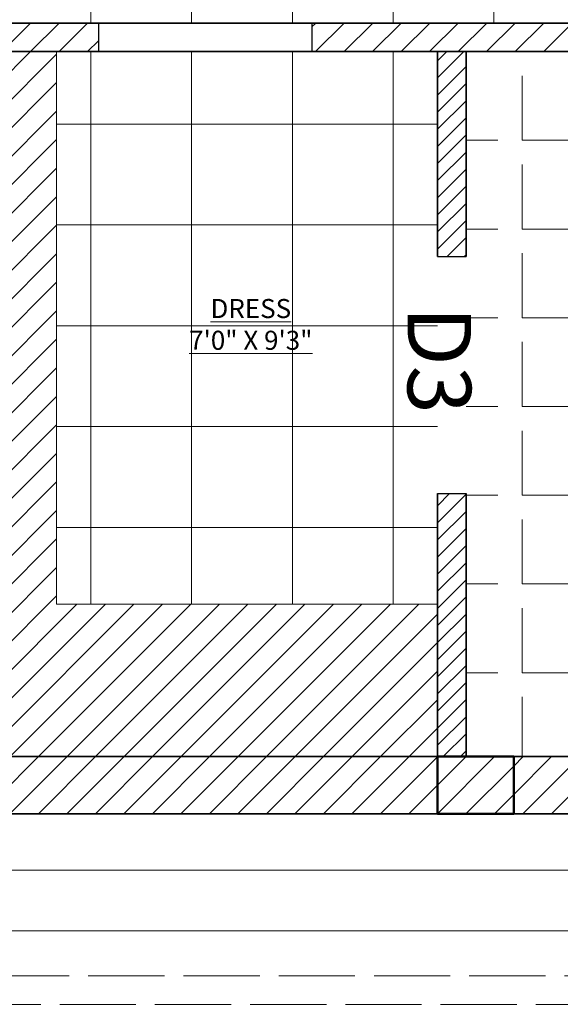
# Model space of a CAD drawing. Units: inches. Extents: x 2036 to 2670, y 319 to 920.
# Tile 12 of 15: x 2449 to 2535, y 465 to 620. Entities that reach past the tile are written whole.
import ezdxf

# ---------------------------------------------------------------- set-up
doc = ezdxf.new("R2010")
doc.units = ezdxf.units.IN
doc.linetypes.add('ACAD_ISO02W100', pattern=[15, 12, -3])
for name, color, linetype, lineweight in [('A-ANNO-DIMS', 2, 'Continuous', 18), ('A-ANNO-TEXT', 7, 'Continuous', 18), ('A-AREA-IDEN', 7, 'Continuous', 18), ('A-CASE', 7, 'Continuous', 18), ('A-CASE-PATT', 9, 'Continuous', 13), ('A-COLS', 7, 'Continuous', 50), ('A-DOOR', 3, 'Continuous', 25), ('A-FLOR-OVHD', 1, 'ACAD_ISO02W100', 13), ('A-FLOR-PATT', 8, 'Continuous', 9), ('A-WALL', 7, 'Continuous', 35)]:
    doc.layers.add(name, color=color, linetype=linetype, lineweight=lineweight)
doc.layers.add('A-COLS-PATT', color=240, linetype='Continuous', lineweight=13, true_color=0xed1f24)
doc.layers.add('A-WALL-PATT', color=52, linetype='Continuous', lineweight=13, true_color=0xc8c92d)
doc.styles.get("Standard").update_dxf_attribs({"font": 'arial.ttf'})
doc.dimstyles.new('ISO-25', dxfattribs={"dimtxt": 10, "dimasz": 6, "dimexe": 1.25, "dimexo": 0.625, "dimtad": 0, "dimdec": 1, "dimlunit": 3, "dimtxsty": 'Standard', "dimblk": 'OBLIQUE', "dimcen": 2.5, "dimclrd": 94, "dimclre": 94, "dimclrt": 1, "dimadec": 0, "dimazin": 0, "dimtfac": 1, "dimtdec": 1, "dimtmove": 0, "dimatfit": 3, "dimfxl": 1, "dimfxlon": 1, "dimarcsym": 0})

# ---------------------------------------------------------------- blocks, each defined once
blk = doc.blocks.new('COL-9x12')
blk.add_lwpolyline([(9, 0), (0, 0), (0, 12), (9, 12)], close=True)
blk = doc.blocks.new('_Oblique')
at = {"color": 0, "linetype": 'ByBlock', "lineweight": -2}
blk.add_line((-0.5, -0.5), (0.5, 0.5), dxfattribs=at)
blk = doc.blocks.new('*D54')
at = {"layer": 'A-ANNO-DIMS', "color": 94, "lineweight": -2, "transparency": 16777216}
for p, q in [((2642.09, 545.51), (2642.09, 551.51)), ((2641.09, 545.51), (2643.34, 545.51)), ((2642.09, 513.19), (2642.09, 545.51)), ((2641.09, 513.19), (2643.34, 513.19))]:
    blk.add_line(p, q, dxfattribs=at)
at = {"layer": 'Defpoints', "color": 0, "transparency": 16777216}
for p in [(2158.74, 545.51), (2642.09, 545.51), (2158.74, 513.19)]:
    blk.add_point(p, dxfattribs=at)
at = {"layer": 'A-ANNO-DIMS', "color": 94, "lineweight": -2, "transparency": 16777216, "xscale": 6, "yscale": 6, "zscale": 6}
for p, rotation in [((2642.09, 545.51), 90), ((2642.09, 513.19), 270)]:
    blk.add_blockref('_Oblique', p, dxfattribs=dict(at, rotation=rotation))
at = {"layer": 'A-ANNO-DIMS', "color": 1, "transparency": 16777216, "insert": (2642.09, 577.16), "char_height": 10, "attachment_point": 5, "rotation": 90}
blk.add_mtext('2\'-8 1/2"', dxfattribs=at)
blk = doc.blocks.new('*D55')
at = {"layer": 'A-ANNO-DIMS', "color": 94, "lineweight": -2, "transparency": 16777216}
for p, q in [((2641.09, 582.53), (2643.34, 582.53)), ((2642.09, 582.53), (2642.09, 577.94)), ((2642.09, 545.51), (2642.09, 550.11)), ((2641.09, 545.51), (2643.34, 545.51))]:
    blk.add_line(p, q, dxfattribs=at)
at = {"layer": 'Defpoints', "color": 0, "transparency": 16777216}
for p in [(2158.74, 582.53), (2642.09, 582.53), (2158.74, 545.51)]:
    blk.add_point(p, dxfattribs=at)
at = {"layer": 'A-ANNO-DIMS', "color": 94, "lineweight": -2, "transparency": 16777216, "xscale": 6, "yscale": 6, "zscale": 6}
for p, rotation in [((2642.09, 582.53), 90), ((2642.09, 545.51), 270)]:
    blk.add_blockref('_Oblique', p, dxfattribs=dict(at, rotation=rotation))
at = {"layer": 'A-ANNO-DIMS', "color": 1, "transparency": 16777216, "insert": (2642.09, 564.02), "char_height": 10, "attachment_point": 5, "rotation": 90}
blk.add_mtext('3\'-1"', dxfattribs=at)
blk = doc.blocks.new('*D56')
at = {"layer": 'A-ANNO-DIMS', "color": 94, "lineweight": -2, "transparency": 16777216}
for p, q in [((2642.09, 599.85), (2642.09, 605.85)), ((2641.09, 599.85), (2643.34, 599.85)), ((2642.09, 582.53), (2642.09, 599.85)), ((2641.09, 582.53), (2643.34, 582.53))]:
    blk.add_line(p, q, dxfattribs=at)
at = {"layer": 'Defpoints', "color": 0, "transparency": 16777216}
for p in [(2158.74, 599.85), (2642.09, 599.85), (2158.74, 582.53)]:
    blk.add_point(p, dxfattribs=at)
at = {"layer": 'A-ANNO-DIMS', "color": 94, "lineweight": -2, "transparency": 16777216, "xscale": 6, "yscale": 6, "zscale": 6}
for p, rotation in [((2642.09, 599.85), 90), ((2642.09, 582.53), 270)]:
    blk.add_blockref('_Oblique', p, dxfattribs=dict(at, rotation=rotation))
at = {"layer": 'A-ANNO-DIMS', "color": 1, "transparency": 16777216, "insert": (2642.09, 630.95), "char_height": 10, "attachment_point": 5, "rotation": 90}
blk.add_mtext('1\'-5 1/2"', dxfattribs=at)
blk = doc.blocks.new('*D60')
at = {"layer": 'A-ANNO-DIMS', "color": 94, "lineweight": -2, "transparency": 16777216}
for p, q in [((2051.39, 582.41), (2051.39, 588.41)), ((2052.39, 582.41), (2050.14, 582.41)), ((2051.39, 545.09), (2051.39, 582.41)), ((2052.39, 545.09), (2050.14, 545.09))]:
    blk.add_line(p, q, dxfattribs=at)
at = {"layer": 'Defpoints', "color": 0, "transparency": 16777216}
for p in [(2051.39, 582.41), (2515.24, 582.41), (2515.24, 545.09)]:
    blk.add_point(p, dxfattribs=at)
at = {"layer": 'A-ANNO-DIMS', "color": 94, "lineweight": -2, "transparency": 16777216, "xscale": 6, "yscale": 6, "zscale": 6}
for p, rotation in [((2051.39, 582.41), 90), ((2051.39, 545.09), 270)]:
    blk.add_blockref('_Oblique', p, dxfattribs=dict(at, rotation=rotation))
at = {"layer": 'A-ANNO-DIMS', "color": 1, "transparency": 16777216, "insert": (2051.39, 613.98), "char_height": 10, "attachment_point": 5, "rotation": 90}
blk.add_mtext('3\'-1 1/2"', dxfattribs=at)

msp = doc.modelspace()

# ---------------------------------------------------------------- hatches: boundary and pattern name
at = {"layer": 'A-CASE-PATT'}
h = msp.add_hatch(dxfattribs=at)
h.set_pattern_fill('ANSI31', color=256)
h.paths.add_polyline_path([(2455.24, 614.68), (2431.24, 614.68), (2431.24, 503.68), (2515.24, 503.68), (2515.24, 527.68), (2455.24, 527.68)])
at = {"layer": 'A-COLS-PATT'}
h = msp.add_hatch(dxfattribs=at)
h.set_pattern_fill('ANSI31', color=256)
h.paths.add_polyline_path([(2089.74, 875.68), (2080.74, 875.68), (2080.74, 863.68), (2089.74, 863.68)])
h.paths.add_polyline_path([(2089.74, 821.68), (2080.74, 821.68), (2080.74, 809.68), (2089.74, 809.68)])
h.paths.add_polyline_path([(2089.74, 624.2), (2080.74, 624.2), (2080.74, 612.2), (2089.74, 612.2)])
h.paths.add_polyline_path([(2158.74, 506.68), (2149.74, 506.68), (2149.74, 494.68), (2158.74, 494.68)])
h.paths.add_polyline_path([(2158.74, 617.33), (2149.74, 617.33), (2149.74, 605.33), (2158.74, 605.33)])
h.paths.add_polyline_path([(2158.74, 736.18), (2149.74, 736.18), (2149.74, 724.18), (2158.74, 724.18)])
h.paths.add_polyline_path([(2158.74, 852.81), (2149.74, 852.81), (2149.74, 843.81), (2158.74, 843.81)])
h.paths.add_polyline_path([(2161.74, 852.81), (2158.74, 852.81), (2158.74, 843.81), (2161.74, 843.81)])
h.paths.add_polyline_path([(2295.21, 857.66), (2290.74, 857.66), (2290.74, 848.68), (2295.21, 848.68)])
h.paths.add_polyline_path([(2290.74, 857.66), (2283.21, 857.66), (2283.21, 848.66), (2290.74, 848.66)])
h.paths.add_polyline_path([(2443.62, 857.68), (2431.62, 857.68), (2431.62, 848.68), (2443.62, 848.68)])
h.paths.add_polyline_path([(2561.81, 857.68), (2549.81, 857.68), (2549.81, 848.68), (2561.81, 848.68)])
h.paths.add_polyline_path([(2295.24, 737.65), (2290.74, 737.65), (2290.74, 728.68), (2295.24, 728.68)])
h.paths.add_polyline_path([(2309.27, 612.12), (2297.27, 612.12), (2297.27, 603.12), (2309.27, 603.12)])
h.paths.add_polyline_path([(2282.24, 503.68), (2270.24, 503.68), (2270.24, 494.68), (2282.24, 494.68)])
h.paths.add_polyline_path([(2431.74, 746.09), (2427.24, 746.09), (2427.24, 737.09), (2431.74, 737.09)])
h.paths.add_polyline_path([(2439.24, 746.09), (2431.74, 746.09), (2431.74, 737.09), (2439.24, 737.09)])
h.paths.add_polyline_path([(2596.59, 736.59), (2584.59, 736.59), (2584.59, 727.59), (2596.59, 727.59)])
h.paths.add_polyline_path([(2586.39, 623.71), (2574.39, 623.71), (2574.39, 619.18), (2586.39, 619.18)])
h.paths.add_polyline_path([(2586.39, 619.18), (2574.39, 619.18), (2574.39, 614.71), (2586.39, 614.71)])
h.paths.add_polyline_path([(2438.74, 623.68), (2431.24, 623.68), (2431.24, 619.18), (2438.74, 619.18)])
h.paths.add_polyline_path([(2438.74, 619.18), (2431.24, 619.18), (2431.24, 614.68), (2438.74, 614.68)])
h.paths.add_polyline_path([(2431.24, 623.68), (2426.74, 623.68), (2426.74, 614.68), (2431.24, 614.68), (2431.24, 619.18)])
h.paths.add_polyline_path([(2527.24, 503.68), (2515.24, 503.68), (2515.24, 494.68), (2527.24, 494.68)])
h.paths.add_polyline_path([(2590.31, 503.68), (2578.31, 503.68), (2578.31, 494.68), (2590.31, 494.68)])
at = {"layer": 'A-FLOR-PATT'}
h = msp.add_hatch(dxfattribs=at)
h.set_pattern_fill('ANSI31', color=256, scale=5, angle=135)
h.paths.add_polyline_path([(2290.74, 659.68), (2158.74, 659.68), (2158.74, 582.53), (2158.74, 545.51), (2158.74, 503.68), (2426.74, 503.68), (2426.74, 614.68), (2426.74, 623.68), (2426.74, 628.18), (2431.24, 628.18), (2431.24, 623.68), (2438.74, 623.68), (2438.74, 619.18), (2574.39, 619.18), (2574.39, 623.71), (2586.39, 623.71), (2586.39, 619.18), (2603.74, 619.18), (2603.74, 824.68), (2431.74, 824.68), (2431.74, 746.09), (2439.24, 746.09), (2439.24, 737.09), (2431.74, 737.09), (2431.74, 659.68), (2427.24, 659.68), (2427.24, 739.48), (2383.24, 739.48), (2383.24, 804.68), (2339.24, 804.68), (2339.24, 749.08), (2295.24, 749.08), (2295.24, 737.65), (2295.27, 737.65), (2295.27, 728.65), (2295.21, 728.65, -0.586418), (2272.74, 728.68), (2272.74, 824.68), (2270.11, 824.68), (2270.11, 829.18), (2290.74, 829.18), (2290.74, 848.66), (2283.21, 848.66), (2283.21, 857.66), (2289.74, 857.66), (2289.74, 874.68), (2158.74, 874.68), (2158.74, 852.81), (2161.74, 852.81), (2161.74, 843.81), (2158.74, 843.81), (2158.74, 829.18), (2224.74, 829.18), (2224.74, 800.68), (2182.74, 800.68), (2182.74, 733.41), (2158.74, 733.41), (2158.74, 728.68), (2235.24, 728.68), (2235.24, 714.81), (2230.74, 714.81), (2230.74, 724.18), (2158.74, 724.18), (2158.74, 664.18), (2230.74, 664.18), (2230.74, 678.81), (2235.24, 678.81), (2235.24, 664.18), (2290.74, 664.18)])
h.paths.add_polyline_path([(2309.27, 612.12), (2309.27, 603.12), (2297.27, 603.12), (2297.27, 612.12)], flags=16)
h.paths.add_polyline_path([(2280.12, 639.11), (2280.26, 638.18, -0.414214), (2279.26, 637.18), (2278.76, 637.18), (2279.26, 633.18), (2277.76, 633.18), (2277.26, 637.18), (2269.76, 637.18), (2262.26, 637.18), (2261.76, 633.18), (2260.26, 633.18), (2260.76, 637.18), (2260.26, 637.18, -0.414214), (2259.26, 638.18), (2259.41, 639.11, -0.541164), (2257.76, 641.18), (2260.76, 652.18), (2261.45, 652.18), (2261.53, 652.68), (2262.76, 652.68), (2262.25, 655.24, 0.001913), (2261.76, 655.18), (2259.76, 658.18, -0.15), (2279.76, 658.18), (2277.76, 655.18, 0.001913), (2277.27, 655.24), (2276.76, 652.68), (2278, 652.68), (2278.07, 652.18), (2278.76, 652.18), (2281.76, 641.18, -0.541163)], flags=16)
h.paths.add_polyline_path([(2245.98, 639.11), (2246.13, 638.18, -0.414214), (2245.13, 637.18), (2244.63, 637.18), (2245.13, 633.18), (2243.63, 633.18), (2243.13, 637.18), (2235.63, 637.18), (2228.13, 637.18), (2227.63, 633.18), (2226.13, 633.18), (2226.63, 637.18), (2226.13, 637.18, -0.414214), (2225.13, 638.18), (2225.27, 639.11, -0.541164), (2223.63, 641.18), (2226.63, 652.18), (2227.32, 652.18), (2227.39, 652.68), (2228.63, 652.68), (2228.12, 655.24, 0.001913), (2227.63, 655.18), (2225.63, 658.18, -0.15), (2245.63, 658.18), (2243.63, 655.18, 0.001913), (2243.14, 655.24), (2242.63, 652.68), (2243.86, 652.68), (2243.94, 652.18), (2244.63, 652.18), (2247.63, 641.18, -0.541163)], flags=16)
h.paths.add_polyline_path([(2351.59, 515.15, -0.151948), (2279.59, 515.15), (2279.59, 537.68), (2273.59, 537.68), (2273.59, 511.68, 0.190476), (2357.59, 511.68), (2357.59, 537.68), (2351.59, 537.68)])
h.paths.add_polyline_path([(2327.59, 536.13), (2327.59, 517.07), (2303.59, 517.07), (2303.59, 536.13)], flags=16)
h.paths.add_polyline_path([(2213.4, 639.11), (2213.55, 638.18, -0.414214), (2212.55, 637.18), (2212.05, 637.18), (2212.55, 633.18), (2211.05, 633.18), (2210.55, 637.18), (2203.05, 637.18), (2195.55, 637.18), (2195.05, 633.18), (2193.55, 633.18), (2194.05, 637.18), (2193.55, 637.18, -0.414214), (2192.55, 638.18), (2192.69, 639.11, -0.541164), (2191.05, 641.18), (2194.05, 652.18), (2194.73, 652.18), (2194.81, 652.68), (2196.05, 652.68), (2195.53, 655.24, 0.001913), (2195.05, 655.18), (2193.05, 658.18, -0.15), (2213.05, 658.18), (2211.05, 655.18, 0.001913), (2210.56, 655.24), (2210.05, 652.68), (2211.28, 652.68), (2211.36, 652.18), (2212.05, 652.18), (2215.05, 641.18, -0.541163)], flags=16)
h.paths.add_polyline_path([(2368.58, 538.02), (2370.52, 538.02), (2371.17, 532.84), (2380.89, 532.84), (2390.6, 532.84), (2391.25, 538.02), (2393.2, 538.02), (2392.55, 532.84), (2380.89, 532.84), (2368.58, 532.84, 0.414214), (2367.28, 531.54), (2367.47, 530.34, -0.483352), (2369.23, 527.65), (2371.82, 513.4), (2370.12, 513.4), (2370.22, 512.75), (2391.56, 512.75), (2391.66, 513.4), (2389.96, 513.4), (2392.55, 527.65, -1.387427), (2396.43, 527.65), (2392.55, 513.4), (2391.66, 513.4), (2391.56, 512.75), (2389.31, 512.75), (2390, 509.37, 0.003796), (2391.25, 509.51), (2393.84, 505.63, -0.15), (2367.93, 505.63), (2370.52, 509.51, 0.003901), (2371.81, 509.36), (2372.47, 512.75), (2370.22, 512.75), (2370.12, 513.4), (2369.23, 513.4), (2365.34, 527.65, -0.541163), (2367.47, 530.34), (2367.28, 531.54, -0.414214), (2368.58, 532.84), (2369.23, 532.84)])
h.paths.add_polyline_path([(2266.74, 538.02), (2266.09, 532.84), (2254.43, 532.84), (2242.12, 532.84, 0.414214), (2240.83, 531.54), (2241.01, 530.34, -0.483352), (2242.77, 527.65), (2245.36, 513.4), (2243.66, 513.4), (2243.76, 512.75), (2265.1, 512.75), (2265.2, 513.4), (2263.5, 513.4), (2266.09, 527.65, -1.387427), (2269.98, 527.65), (2266.09, 513.4), (2265.2, 513.4), (2265.1, 512.75), (2262.85, 512.75), (2263.54, 509.37, 0.003796), (2264.79, 509.51), (2267.39, 505.63, -0.15), (2241.47, 505.63), (2244.07, 509.51, 0.003901), (2245.36, 509.36), (2246.01, 512.75), (2243.76, 512.75), (2243.66, 513.4), (2242.77, 513.4), (2238.88, 527.65, -0.541163), (2241.01, 530.34), (2240.83, 531.54, -0.414214), (2242.12, 532.84), (2242.77, 532.84), (2242.12, 538.02), (2244.07, 538.02), (2244.71, 532.84), (2254.43, 532.84), (2264.15, 532.84), (2264.79, 538.02)])
h.paths.add_polyline_path([(2185.24, 620.36), (2185.24, 618.86), (2181.24, 618.36), (2181.24, 610.86), (2181.24, 603.36), (2185.24, 602.86), (2185.24, 601.36), (2181.24, 601.86), (2181.24, 601.36, -0.414214), (2180.24, 600.36), (2179.31, 600.5, -0.541164), (2177.24, 598.86), (2166.24, 601.86), (2166.24, 602.54), (2165.74, 602.62), (2165.74, 603.86), (2163.18, 603.34, 0.001913), (2163.24, 602.86), (2160.24, 600.86, -0.15), (2160.24, 620.86), (2163.24, 618.86, 0.001913), (2163.18, 618.37), (2165.74, 617.86), (2165.74, 619.09), (2166.24, 619.17), (2166.24, 619.86), (2177.24, 622.86, -0.541163), (2179.31, 621.21), (2180.24, 621.36, -0.414214), (2181.24, 620.36), (2181.24, 619.86)])
h.paths.add_polyline_path([(2470.92, 676.01), (2470.92, 806.13), (2568.52, 806.13), (2568.52, 676.01)], flags=16)
h.paths.add_polyline_path([(2177.74, 677.49), (2161.9, 677.49), (2161.9, 705.85), (2177.74, 705.85)], flags=16)
h.paths.add_polyline_path([(2176.74, 678.49), (2162.9, 678.49), (2162.9, 704.85), (2176.74, 704.85)], flags=0)
h.paths.add_polyline_path([(2175.01, 686.48), (2172.93, 686.48), (2172.93, 690.63), (2170.86, 690.63), (2170.86, 686.48), (2164.63, 686.48), (2164.63, 688.56), (2166.71, 688.56), (2168.78, 688.56), (2168.78, 690.63), (2164.63, 690.63), (2164.63, 696.85), (2166.71, 696.85), (2166.71, 692.71), (2168.78, 692.71), (2168.78, 696.85), (2175.01, 696.85), (2175.01, 694.78), (2170.86, 694.78), (2170.86, 692.71), (2175.01, 692.71)], flags=0)
h.paths.add_polyline_path([(2543.79, 782.71), (2483.94, 782.71), (2483.94, 804.18), (2517.77, 804.18), (2517.77, 782.71), (2521.67, 782.71), (2521.67, 804.18), (2555.5, 804.18), (2555.5, 779.45), (2547.05, 779.45), (2568.52, 757.98), (2543.79, 757.98)], flags=0)
h.paths.add_polyline_path([(2584.59, 727.59), (2584.59, 736.59), (2596.59, 736.59), (2596.59, 727.59)], flags=16)
h.paths.add_polyline_path([(2520.45, 647.03), (2553.79, 647.03), (2553.79, 658.23), (2520.45, 658.23)], flags=24)
h.paths.add_polyline_path([(2299.53, 573.74), (2331.71, 573.74), (2331.71, 584.94), (2299.53, 584.94)], flags=24)
h.paths.add_polyline_path([(2191.59, 685.19), (2212.12, 685.19), (2212.12, 696.38), (2191.59, 696.38)], flags=24)
h.paths.add_polyline_path([(2353.9, 649.86), (2379.08, 649.86), (2379.08, 661.06), (2353.9, 661.06)], flags=24)
h.paths.add_polyline_path([(2214.61, 763.31), (2237.46, 763.31), (2237.46, 779.56), (2214.61, 779.56)], flags=24)
h.paths.add_polyline_path([(2225.09, 819.31), (2269.29, 819.31), (2269.29, 844.04), (2225.09, 844.04)], flags=24)
h.paths.add_polyline_path([(2204.06, 845.04), (2226.92, 845.04), (2226.92, 856.24), (2204.06, 856.24)], flags=24)
h = msp.add_hatch(dxfattribs=at)
h.set_pattern_fill('ANSI31', color=256, scale=5, angle=45)
h.paths.add_polyline_path([(2290.74, 659.68), (2158.74, 659.68), (2158.74, 582.53), (2158.74, 545.51), (2158.74, 503.68), (2426.74, 503.68), (2426.74, 614.68), (2426.74, 623.68), (2426.74, 628.18), (2431.24, 628.18), (2431.24, 623.68), (2438.74, 623.68), (2438.74, 619.18), (2574.39, 619.18), (2574.39, 623.71), (2586.39, 623.71), (2586.39, 619.18), (2603.74, 619.18), (2603.74, 824.68), (2431.74, 824.68), (2431.74, 746.09), (2439.24, 746.09), (2439.24, 737.09), (2431.74, 737.09), (2431.74, 659.68), (2427.24, 659.68), (2427.24, 739.48), (2383.24, 739.48), (2383.24, 804.68), (2339.24, 804.68), (2339.24, 749.08), (2295.24, 749.08), (2295.24, 737.65), (2295.27, 737.65), (2295.27, 728.65), (2295.21, 728.65, -0.586418), (2272.74, 728.68), (2272.74, 824.68), (2270.11, 824.68), (2270.11, 829.18), (2290.74, 829.18), (2290.74, 848.66), (2283.21, 848.66), (2283.21, 857.66), (2289.74, 857.66), (2289.74, 874.68), (2158.74, 874.68), (2158.74, 852.81), (2161.74, 852.81), (2161.74, 843.81), (2158.74, 843.81), (2158.74, 829.18), (2224.74, 829.18), (2224.74, 800.68), (2182.74, 800.68), (2182.74, 733.41), (2158.74, 733.41), (2158.74, 728.68), (2235.24, 728.68), (2235.24, 714.81), (2230.74, 714.81), (2230.74, 724.18), (2158.74, 724.18), (2158.74, 664.18), (2230.74, 664.18), (2230.74, 678.81), (2235.24, 678.81), (2235.24, 664.18), (2290.74, 664.18)])
h.paths.add_polyline_path([(2309.27, 612.12), (2309.27, 603.12), (2297.27, 603.12), (2297.27, 612.12)], flags=16)
h.paths.add_polyline_path([(2280.12, 639.11), (2280.26, 638.18, -0.414214), (2279.26, 637.18), (2278.76, 637.18), (2279.26, 633.18), (2277.76, 633.18), (2277.26, 637.18), (2269.76, 637.18), (2262.26, 637.18), (2261.76, 633.18), (2260.26, 633.18), (2260.76, 637.18), (2260.26, 637.18, -0.414214), (2259.26, 638.18), (2259.41, 639.11, -0.541164), (2257.76, 641.18), (2260.76, 652.18), (2261.45, 652.18), (2261.53, 652.68), (2262.76, 652.68), (2262.25, 655.24, 0.001913), (2261.76, 655.18), (2259.76, 658.18, -0.15), (2279.76, 658.18), (2277.76, 655.18, 0.001913), (2277.27, 655.24), (2276.76, 652.68), (2278, 652.68), (2278.07, 652.18), (2278.76, 652.18), (2281.76, 641.18, -0.541163)], flags=16)
h.paths.add_polyline_path([(2245.98, 639.11), (2246.13, 638.18, -0.414214), (2245.13, 637.18), (2244.63, 637.18), (2245.13, 633.18), (2243.63, 633.18), (2243.13, 637.18), (2235.63, 637.18), (2228.13, 637.18), (2227.63, 633.18), (2226.13, 633.18), (2226.63, 637.18), (2226.13, 637.18, -0.414214), (2225.13, 638.18), (2225.27, 639.11, -0.541164), (2223.63, 641.18), (2226.63, 652.18), (2227.32, 652.18), (2227.39, 652.68), (2228.63, 652.68), (2228.12, 655.24, 0.001913), (2227.63, 655.18), (2225.63, 658.18, -0.15), (2245.63, 658.18), (2243.63, 655.18, 0.001913), (2243.14, 655.24), (2242.63, 652.68), (2243.86, 652.68), (2243.94, 652.18), (2244.63, 652.18), (2247.63, 641.18, -0.541163)], flags=16)
h.paths.add_polyline_path([(2351.59, 537.68), (2351.59, 515.15, -0.151948), (2279.59, 515.15), (2279.59, 537.68), (2273.59, 537.68), (2273.59, 511.68, 0.190476), (2357.59, 511.68), (2357.59, 537.68)])
h.paths.add_polyline_path([(2368.58, 538.02), (2370.52, 538.02), (2371.17, 532.84), (2380.89, 532.84), (2390.6, 532.84), (2391.25, 538.02), (2393.2, 538.02), (2392.55, 532.84), (2380.89, 532.84), (2368.58, 532.84, 0.414214), (2367.28, 531.54), (2367.47, 530.34, -0.483352), (2369.23, 527.65), (2371.82, 513.4), (2370.12, 513.4), (2370.22, 512.75), (2391.56, 512.75), (2391.66, 513.4), (2389.96, 513.4), (2392.55, 527.65, -1.387427), (2396.43, 527.65), (2392.55, 513.4), (2391.66, 513.4), (2391.56, 512.75), (2389.31, 512.75), (2390, 509.37, 0.003796), (2391.25, 509.51), (2393.84, 505.63, -0.15), (2367.93, 505.63), (2370.52, 509.51, 0.003901), (2371.81, 509.36), (2372.47, 512.75), (2370.22, 512.75), (2370.12, 513.4), (2369.23, 513.4), (2365.34, 527.65, -0.541163), (2367.47, 530.34), (2367.28, 531.54, -0.414214), (2368.58, 532.84), (2369.23, 532.84)])
h.paths.add_polyline_path([(2327.59, 536.13), (2327.59, 517.07), (2303.59, 517.07), (2303.59, 536.13)], flags=16)
h.paths.add_polyline_path([(2470.92, 676.01), (2470.92, 806.13), (2568.52, 806.13), (2568.52, 676.01)], flags=16)
h.paths.add_polyline_path([(2266.74, 538.02), (2266.09, 532.84), (2254.43, 532.84), (2242.12, 532.84, 0.414214), (2240.83, 531.54), (2241.01, 530.34, -0.483352), (2242.77, 527.65), (2245.36, 513.4), (2243.66, 513.4), (2243.76, 512.75), (2265.1, 512.75), (2265.2, 513.4), (2263.5, 513.4), (2266.09, 527.65, -1.387427), (2269.98, 527.65), (2266.09, 513.4), (2265.2, 513.4), (2265.1, 512.75), (2262.85, 512.75), (2263.54, 509.37, 0.003796), (2264.79, 509.51), (2267.39, 505.63, -0.15), (2241.47, 505.63), (2244.07, 509.51, 0.003901), (2245.36, 509.36), (2246.01, 512.75), (2243.76, 512.75), (2243.66, 513.4), (2242.77, 513.4), (2238.88, 527.65, -0.541163), (2241.01, 530.34), (2240.83, 531.54, -0.414214), (2242.12, 532.84), (2242.77, 532.84), (2242.12, 538.02), (2244.07, 538.02), (2244.71, 532.84), (2254.43, 532.84), (2264.15, 532.84), (2264.79, 538.02)])
h.paths.add_polyline_path([(2213.4, 639.11), (2213.55, 638.18, -0.414214), (2212.55, 637.18), (2212.05, 637.18), (2212.55, 633.18), (2211.05, 633.18), (2210.55, 637.18), (2203.05, 637.18), (2195.55, 637.18), (2195.05, 633.18), (2193.55, 633.18), (2194.05, 637.18), (2193.55, 637.18, -0.414214), (2192.55, 638.18), (2192.69, 639.11, -0.541164), (2191.05, 641.18), (2194.05, 652.18), (2194.73, 652.18), (2194.81, 652.68), (2196.05, 652.68), (2195.53, 655.24, 0.001913), (2195.05, 655.18), (2193.05, 658.18, -0.15), (2213.05, 658.18), (2211.05, 655.18, 0.001913), (2210.56, 655.24), (2210.05, 652.68), (2211.28, 652.68), (2211.36, 652.18), (2212.05, 652.18), (2215.05, 641.18, -0.541163)], flags=16)
h.paths.add_polyline_path([(2185.24, 620.36), (2185.24, 618.86), (2181.24, 618.36), (2181.24, 610.86), (2181.24, 603.36), (2185.24, 602.86), (2185.24, 601.36), (2181.24, 601.86), (2181.24, 601.36, -0.414214), (2180.24, 600.36), (2179.31, 600.5, -0.541164), (2177.24, 598.86), (2166.24, 601.86), (2166.24, 602.54), (2165.74, 602.62), (2165.74, 603.86), (2163.18, 603.34, 0.001913), (2163.24, 602.86), (2160.24, 600.86, -0.15), (2160.24, 620.86), (2163.24, 618.86, 0.001913), (2163.18, 618.37), (2165.74, 617.86), (2165.74, 619.09), (2166.24, 619.17), (2166.24, 619.86), (2177.24, 622.86, -0.541163), (2179.31, 621.21), (2180.24, 621.36, -0.414214), (2181.24, 620.36), (2181.24, 619.86)])
h.paths.add_polyline_path([(2177.74, 677.49), (2161.9, 677.49), (2161.9, 705.85), (2177.74, 705.85)], flags=16)
h.paths.add_polyline_path([(2176.74, 678.49), (2162.9, 678.49), (2162.9, 704.85), (2176.74, 704.85)], flags=0)
h.paths.add_polyline_path([(2175.01, 686.48), (2172.93, 686.48), (2172.93, 690.63), (2170.86, 690.63), (2170.86, 686.48), (2164.63, 686.48), (2164.63, 688.56), (2166.71, 688.56), (2168.78, 688.56), (2168.78, 690.63), (2164.63, 690.63), (2164.63, 696.85), (2166.71, 696.85), (2166.71, 692.71), (2168.78, 692.71), (2168.78, 696.85), (2175.01, 696.85), (2175.01, 694.78), (2170.86, 694.78), (2170.86, 692.71), (2175.01, 692.71)], flags=0)
h.paths.add_polyline_path([(2543.79, 782.71), (2483.94, 782.71), (2483.94, 804.18), (2517.77, 804.18), (2517.77, 782.71), (2521.67, 782.71), (2521.67, 804.18), (2555.5, 804.18), (2555.5, 779.45), (2547.05, 779.45), (2568.52, 757.98), (2543.79, 757.98)], flags=0)
h.paths.add_polyline_path([(2584.59, 727.59), (2584.59, 736.59), (2596.59, 736.59), (2596.59, 727.59)], flags=16)
h.paths.add_polyline_path([(2520.45, 647.03), (2553.79, 647.03), (2553.79, 658.23), (2520.45, 658.23)], flags=24)
h.paths.add_polyline_path([(2299.53, 573.74), (2331.71, 573.74), (2331.71, 584.94), (2299.53, 584.94)], flags=24)
h.paths.add_polyline_path([(2191.59, 685.19), (2212.12, 685.19), (2212.12, 696.38), (2191.59, 696.38)], flags=24)
h.paths.add_polyline_path([(2353.9, 649.86), (2379.08, 649.86), (2379.08, 661.06), (2353.9, 661.06)], flags=24)
h.paths.add_polyline_path([(2214.61, 763.31), (2237.46, 763.31), (2237.46, 779.56), (2214.61, 779.56)], flags=24)
h.paths.add_polyline_path([(2225.09, 819.31), (2269.29, 819.31), (2269.29, 844.04), (2225.09, 844.04)], flags=24)
h.paths.add_polyline_path([(2204.06, 845.04), (2226.92, 845.04), (2226.92, 856.24), (2204.06, 856.24)], flags=24)
h = msp.add_hatch(dxfattribs=at)
h.set_pattern_fill('ANSI31', color=256, scale=3, angle=135)
h.paths.add_polyline_path([(2149.74, 582.53), (2149.74, 707.68), (2120.74, 707.68), (2120.74, 599.68, -1), (2118.74, 599.68), (2085.24, 599.68), (2085.24, 506.68), (2089.74, 506.68), (2089.74, 494.68), (2085.24, 494.68), (2085.24, 469.18), (2608.24, 469.18), (2608.24, 494.68), (2149.74, 494.68), (2149.74, 506.68), (2149.74, 545.51)])
h.paths.add_polyline_path([(2143.58, 686.71), (2149.03, 686.71), (2149.03, 692.89), (2143.58, 692.89)], flags=24)
h.paths.add_polyline_path([(2125.99, 700.31), (2133.31, 700.31), (2133.31, 706.49), (2125.99, 706.49)], flags=24)
h = msp.add_hatch(dxfattribs=at)
h.set_pattern_fill('ANSI31', color=256, scale=5, angle=45)
h.paths.add_polyline_path([(2515.24, 614.68), (2455.24, 614.68), (2455.24, 527.68), (2515.24, 527.68)])
h.paths.add_polyline_path([(2475.58, 566.03), (2496.1, 566.03), (2496.1, 577.23), (2475.58, 577.23)], flags=24)
h = msp.add_hatch(dxfattribs=at)
h.set_pattern_fill('ANSI31', color=256, scale=5, angle=135)
h.paths.add_polyline_path([(2515.24, 614.68), (2455.24, 614.68), (2455.24, 527.68), (2515.24, 527.68)])
h.paths.add_polyline_path([(2475.58, 566.03), (2496.1, 566.03), (2496.1, 577.23), (2475.58, 577.23)], flags=24)
h = msp.add_hatch(dxfattribs=at)
h.set_pattern_fill('ANGLE', color=256, scale=2)
h.set_pattern_definition([(0, (0, 0), (0, 13.97), [10.16, -3.81]), (90, (0, 0), (-13.97, 9e-16), [10.16, -3.81])])
h.paths.add_polyline_path([(2519.74, 503.68), (2527.24, 503.68), (2603.74, 503.68), (2603.74, 614.68), (2519.74, 614.68)])
h.paths.add_polyline_path([(2569.98, 598.38), (2571.98, 604.38), (2568.98, 604.38), (2568.98, 602.88), (2565.98, 602.88), (2565.98, 603.88), (2567.98, 603.88), (2567.98, 604.38), (2565.48, 604.38), (2565.48, 612.38), (2586.48, 612.38), (2586.48, 604.38), (2579.98, 604.38), (2581.98, 598.38, -0.501323), (2577.03, 579.52, -0.132891), (2574.94, 579.52, -0.501317)], flags=16)
h.paths.add_polyline_path([(2571.98, 598.38), (2579.98, 598.38, -0.48008), (2577.63, 580.86, -0.215004), (2574.34, 580.86, -0.48008)], flags=0)
h.paths.add_polyline_path([(2546.37, 611.78), (2546.37, 613.08), (2543.76, 613.08), (2543.76, 611.78)], flags=16)
h.paths.add_polyline_path([(2543.76, 609.82), (2544.41, 609.82), (2544.41, 611.13), (2545.72, 611.13), (2545.72, 609.82), (2554.18, 609.82, -0.293434), (2556.79, 605.92), (2554.18, 605.92, 0.553806), (2552.88, 607.22), (2546.37, 607.22), (2546.37, 606.24), (2547.02, 606.24, -0.791418), (2548.4, 605.92, -0.791418), (2547.02, 605.59), (2546.57, 605.59, -0.086626), (2547.58, 602.73, 0.107048), (2548.97, 602.01), (2541.81, 602.01), (2541.16, 602.01, -0.159443)], flags=16)
h.paths.add_polyline_path([(2542.38, 605.92, -1), (2543.84, 605.92, -1)], flags=0)
h.paths.add_polyline_path([(2544.66, 605.92, -1), (2546.12, 605.92, -1)], flags=0)
h.paths.add_polyline_path([(2566.48, 606.38), (2566.48, 610.38, -0.5), (2567.48, 611.38), (2584.48, 611.38, -0.5), (2585.48, 610.38), (2585.48, 606.38, -0.5), (2584.48, 605.38), (2567.48, 605.38, -0.5)], flags=0)
h.paths.add_polyline_path([(2552.87, 546.2), (2581.15, 546.2), (2581.15, 557.39), (2552.87, 557.39)], flags=24)
at = {"layer": 'A-WALL-PATT'}
h = msp.add_hatch(dxfattribs=at)
h.set_pattern_fill('ANSI31', color=256)
h.paths.add_polyline_path([(2089.74, 863.68), (2080.74, 863.68), (2080.74, 821.68), (2089.74, 821.68)])
h.paths.add_polyline_path([(2089.74, 809.68), (2080.74, 809.68), (2080.74, 624.2), (2089.74, 624.2), (2089.74, 707.68), (2089.74, 767.68)])
h.paths.add_polyline_path([(2149.74, 818.68), (2089.74, 818.68), (2089.74, 809.68), (2149.74, 809.68)])
h.paths.add_polyline_path([(2158.74, 875.68), (2089.74, 875.68), (2089.74, 866.68), (2149.74, 866.68), (2149.74, 852.81), (2158.74, 852.81)])
h.paths.add_polyline_path([(2158.74, 843.81), (2149.74, 843.81), (2149.74, 736.18), (2158.74, 736.18), (2158.74, 824.68)])
h.paths.add_polyline_path([(2181.31, 829.18), (2158.74, 829.18), (2158.74, 824.68), (2181.31, 824.68)])
h.paths.add_polyline_path([(2224.74, 829.18), (2212.72, 829.18), (2212.72, 824.68), (2224.74, 824.68)])
h.paths.add_polyline_path([(2177.02, 503.68), (2158.74, 503.68), (2158.74, 494.68), (2177.02, 494.68)])
h.paths.add_polyline_path([(2158.74, 664.18), (2158.74, 680.02), (2149.74, 680.02), (2149.74, 617.33), (2158.74, 617.33)])
h.paths.add_polyline_path([(2158.74, 724.18), (2149.74, 724.18), (2149.74, 704.02), (2158.74, 704.02)])
h.paths.add_polyline_path([(2235.24, 728.68), (2158.74, 728.68), (2158.74, 724.18), (2230.74, 724.18), (2230.74, 714.81), (2235.24, 714.81)])
h.paths.add_polyline_path([(2290.74, 664.18), (2235.24, 664.18), (2235.24, 678.81), (2230.74, 678.81), (2230.74, 664.18), (2158.74, 664.18), (2158.74, 659.68), (2290.74, 659.68)])
h.paths.add_polyline_path([(2270.24, 503.68), (2227.17, 503.68), (2227.17, 494.68), (2270.24, 494.68)])
h.paths.add_polyline_path([(2515.24, 503.68), (2380.89, 503.68), (2380.89, 494.68), (2515.24, 494.68)])
h.paths.add_polyline_path([(2292.21, 503.68), (2282.24, 503.68), (2282.24, 494.68), (2292.21, 494.68)])
h.paths.add_polyline_path([(2578.31, 503.68), (2527.24, 503.68), (2527.24, 494.68), (2578.31, 494.68)])
h.paths.add_polyline_path([(2603.74, 503.68), (2590.31, 503.68), (2590.31, 494.68), (2603.74, 494.68)])
h.paths.add_polyline_path([(2612.74, 503.68), (2603.74, 503.68), (2603.74, 494.68), (2612.74, 494.68)])
h.paths.add_polyline_path([(2549.81, 857.68), (2443.62, 857.68), (2443.62, 848.68), (2549.81, 848.68)])
h.paths.add_polyline_path([(2295.24, 848.66), (2290.74, 848.66), (2290.74, 829.18), (2270.11, 829.18), (2270.11, 824.68), (2290.74, 824.68), (2290.74, 737.65), (2295.24, 737.65)])
h.paths.add_polyline_path([(2431.74, 737.09), (2427.24, 737.09), (2427.24, 659.68), (2431.74, 659.68)])
h.paths.add_polyline_path([(2431.74, 848.68), (2427.24, 848.68), (2427.24, 746.09), (2431.74, 746.09)])
h.paths.add_polyline_path([(2574.39, 619.18), (2495.46, 619.18), (2495.46, 614.68), (2574.39, 614.68)])
h.paths.add_polyline_path([(2461.84, 619.18), (2438.74, 619.18), (2438.74, 614.68), (2461.84, 614.68)])
h.paths.add_polyline_path([(2603.74, 619.18), (2586.39, 619.18), (2586.39, 614.68), (2603.74, 614.68)], flags=17)
h = msp.add_hatch(dxfattribs=at)
h.set_pattern_fill('ANSI31', color=256, scale=0.6)
h.paths.add_polyline_path([(2519.74, 614.68), (2515.24, 614.68), (2515.24, 582.41), (2519.74, 582.41)])
h.paths.add_polyline_path([(2519.74, 545.09), (2515.24, 545.09), (2515.24, 503.68), (2519.74, 503.68)])

# ---------------------------------------------------------------- linework, layer by layer
at = {"layer": 'A-CASE'}
for q in [(2455.24, 614.68), (2515.24, 527.68)]:
    msp.add_line((2455.24, 527.68), q, dxfattribs=at)
at = {"layer": 'A-DOOR'}
for p, q in [((2461.84, 619.18), (2461.84, 614.68)), ((2495.46, 619.18), (2495.46, 614.68)), ((2515.24, 582.41), (2519.74, 582.41)), ((2515.24, 545.09), (2519.74, 545.09))]:
    msp.add_line(p, q, dxfattribs=at)
at = {"layer": 'A-FLOR-OVHD'}
for p, q in [((2085.24, 469.18), (2608.24, 469.18)), ((2080.74, 464.68), (2612.74, 464.68))]:
    msp.add_line(p, q, dxfattribs=at)
at = {"layer": 'A-WALL'}
for p, q in [((2603.74, 619.18), (2431.24, 619.18)), ((2603.74, 614.68), (2431.24, 614.68)), ((2515.24, 582.41), (2515.24, 614.68)), ((2519.74, 582.41), (2519.74, 614.68)), ((2515.24, 503.68), (2515.24, 545.09)), ((2519.74, 503.68), (2519.74, 545.09)), ((2227.17, 503.68), (2603.74, 503.68)), ((2227.17, 494.68), (2612.74, 494.68))]:
    msp.add_line(p, q, dxfattribs=at)

# ---------------------------------------------------------------- block references
at = {"layer": 'A-COLS', "rotation": 89.99999999999625}
msp.add_blockref('COL-9x12', (2527.24, 494.68), dxfattribs=at)

# ---------------------------------------------------------------- texts
at = {"layer": 'A-ANNO-TEXT', "insert": (2520.54, 574.6), "char_height": 10, "attachment_point": 1, "rotation": 270}
msp.add_mtext_dynamic_manual_height_columns('D3', width=4.4765, gutter_width=12.5, heights=[0], dxfattribs=at)
at = {"layer": 'A-AREA-IDEN', "insert": (2473.8, 575.73), "char_height": 3, "attachment_point": 1}
msp.add_mtext_dynamic_manual_height_columns('\\pxqc;{\\LDRESS\\P7\'0" X 9\'3"}', width=24.0713, gutter_width=12.5, heights=[0], dxfattribs=at)

# ---------------------------------------------------------------- dimensions: what is measured, and where the dimension line sits
at = {"layer": 'A-ANNO-DIMS'}
for base, p1, p2, picture, middle in [((2642.09, 599.85), (2158.74, 582.53), (2158.74, 599.85), '*D56', (2642.09, 630.95)), ((2051.39, 582.41), (2515.24, 545.09), (2515.24, 582.41), '*D60', (2051.39, 613.98)), ((2642.09, 545.51), (2158.74, 513.19), (2158.74, 545.51), '*D54', (2642.09, 577.16)), ((2642.09, 582.53), (2158.74, 545.51), (2158.74, 582.53), '*D55', (2642.09, 564.02))]:
    dim = msp.add_linear_dim(base=base, p1=p1, p2=p2, angle=90, dimstyle='ISO-25', override={"dimdec": 1, "dimlfac": 1, "dimrnd": 0, "dimzin": 1, "dimdsep": 46, "dimlunit": 4, "dimfrac": 2}, dxfattribs=at)
    dim.commit()
    dim.dimension.update_dxf_attribs({"geometry": picture, "text_midpoint": middle})

doc.saveas('drawing.dxf')
